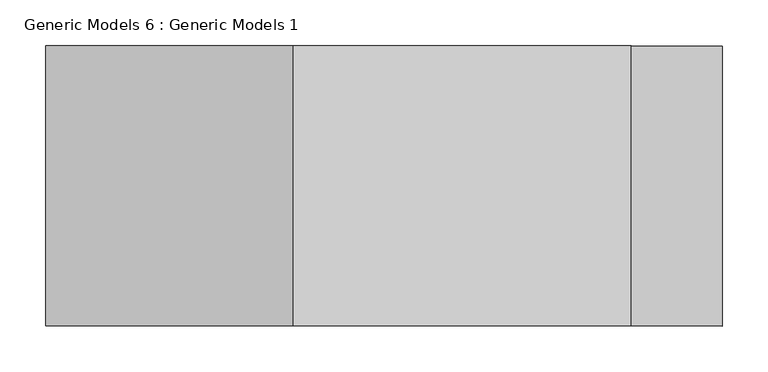
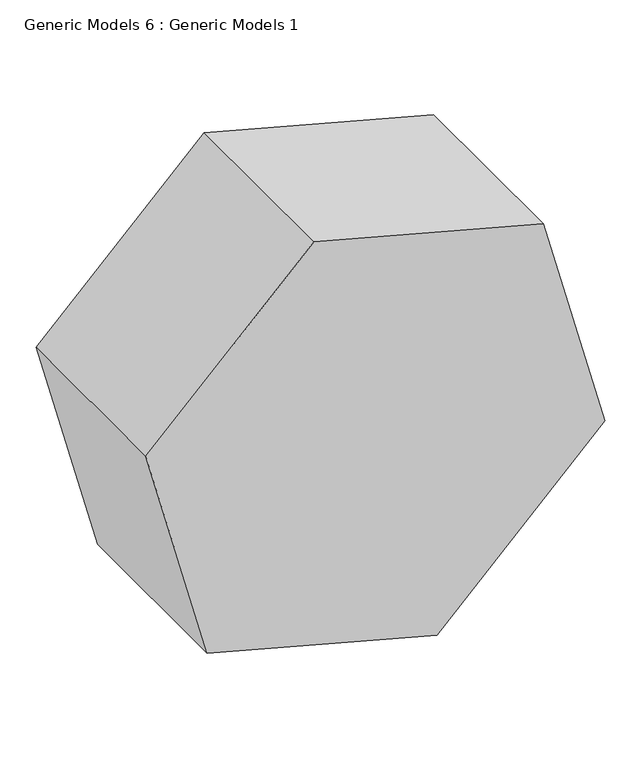
"""IFC4 building model written with IfcOpenShell, lengths in millimetres: proxy geometry, Generic Models 6 : Generic Models 1."""

from ifc_helpers import new_model, si_unit, frame, origin, place, context, project, spatial, polyline, outline, extrude, source, transform, mapped, element, save


def generic_models_6_generic_models_1_19455b19(model_context):
    return source(origin(), model_context, "Body", "SweptSolid", [
        extrude(outline(polyline([(904.7566299, -5377.4070438), (1003.366686, -5745.4247836), (733.9590024, -6014.8324672), (365.9412626, -5916.222411), (267.3312064, -5548.2046712), (536.73889, -5278.7969876), (904.7566299, -5377.4070438)])), frame((0.0, -9086.6225464, 0.0), z_axis=(0.0, 1.0, 0.0), x_axis=(0.0, 0.0, 1.0)), (0.0, 0.0, 1.0), 304.8),
    ])


if __name__ == "__main__":
    model = new_model("IFC4")
    model_context = context("Model", 3, world=origin())
    ifc_project = project(units=[si_unit("LENGTHUNIT", "METRE", prefix="MILLI")], contexts=[model_context])
    site = spatial("IfcSite", under=ifc_project)
    building = spatial("IfcBuilding", under=site)
    placement = place(None, origin())
    generic_models_6_generic_models_1_shape = generic_models_6_generic_models_1_19455b19(model_context)
    element("IfcBuildingElementProxy", 1, Name="Generic Models 6 : Generic Models 1", ObjectType="Generic Models 6 : Generic Models 1", at=placement, inside=building, context=model_context, shape_type="MappedRepresentation", body=[
        mapped(generic_models_6_generic_models_1_shape, transform((0.0, 0.0, 0.0), x_axis=(1.0, 0.0, 0.0), y_axis=(0.0, 1.0, 0.0), z_axis=(0.0, 0.0, 1.0))),
    ])
    save(model, "model.ifc")

# Revit data of these elements
# Element 1 (IfcBuildingElementProxy, "Generic Models 6 : Generic Models 1")
#   Materials on its faces: "Brick, Common"
# Materials
#   "Brick, Common": class "Masonry", colour RGB 170 98 104, transparency 0, Description = "Common brick", Cost = 0
